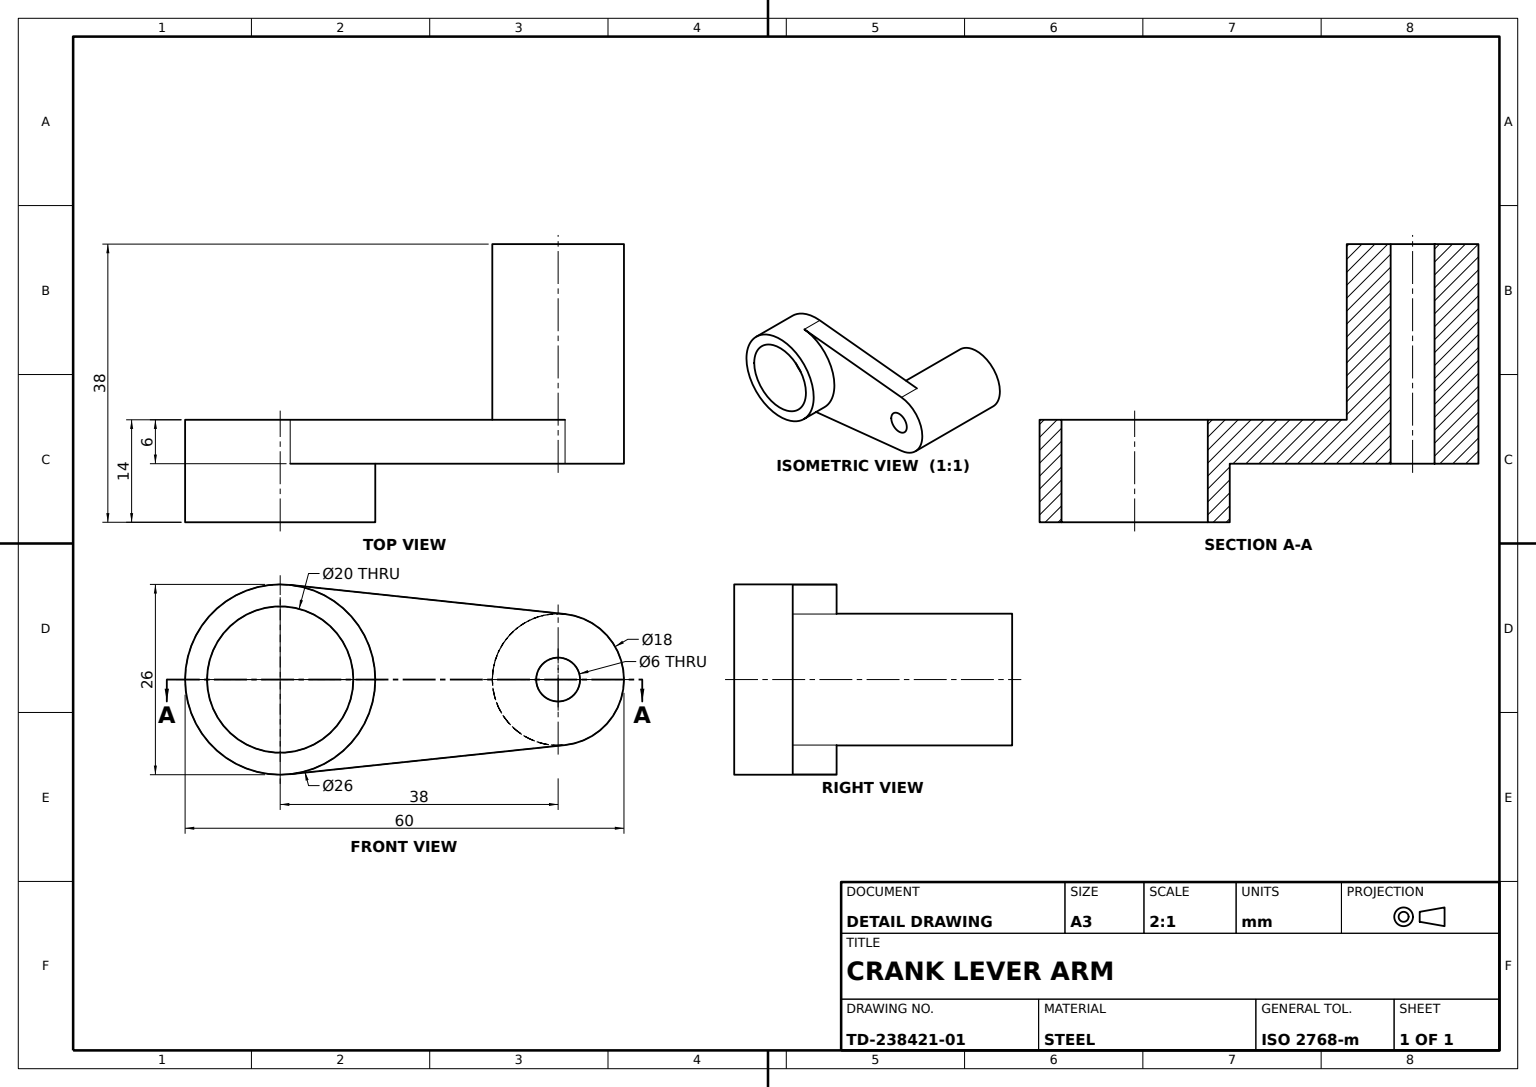
from build123d import *

# Parameters (mm, degrees)
HUB_AND_POST_PROFILE_SKETCH_R   = 13
HUB_AND_POST_PROFILE_SKETCH_R_2 = 10
HUB_RING_26X_20_DEPTH           = 14
SKETCH1_3_R                     = 9
PIN_POST_18_DEPTH               = 24
ARM_WEB_SKETCH_R                = 9
ARM_WEB_6MM_DEPTH               = 6
PIN_HOLE_SKETCH_R               = 3
PIN_HOLE_6_DEPTH                = 37


with BuildPart() as part:
    # Hub and Post Profile Sketch → Hub Ring _26x_20 (new body)
    with BuildSketch(Plane(origin=(0, 0, 0), x_dir=(0, 0, -1), z_dir=(1, 0, 0))):
        Circle(HUB_AND_POST_PROFILE_SKETCH_R)
        Circle(HUB_AND_POST_PROFILE_SKETCH_R_2, mode=Mode.SUBTRACT)
    extrude(amount=HUB_RING_26X_20_DEPTH)



with BuildPart() as body_2:
    # Sketch1_3 → Pin Post _18 (new body)
    with BuildSketch(Plane(origin=(0, 0, 0), x_dir=(0, 0, -1), z_dir=(1, 0, 0))):
        with Locations((38, 0)):
            Circle(SKETCH1_3_R)
    extrude(amount=-PIN_POST_18_DEPTH)


with BuildPart() as part_1:
    add(part.part)

    add(body_2.part)  # Arm Web 6mm merges body 2
    # Arm Web Sketch → Arm Web 6mm (add)
    with BuildSketch(Plane(origin=(0, 0, 0), x_dir=(0, 0, -1), z_dir=(1, 0, 0))):
        with BuildLine():
            Line((38.947368421, 8.949999613), (1.368421053, 12.927777219))
            ThreePointArc((1.368421053, 12.927777219), (9.664095242, 8.695128703), (13, 0))
            ThreePointArc((13, 0), (9.664095242, -8.695128703), (1.368421053, -12.927777219))
            Line((1.368421053, -12.927777219), (38.947368421, -8.949999613))
            ThreePointArc((38.947368421, -8.949999613), (29, 0), (38.947368421, 8.949999613))
        make_face()
        with Locations(Location((38, 0, 0), (0, 0, 276.042328419))):
            Circle(ARM_WEB_SKETCH_R)
    extrude(amount=ARM_WEB_6MM_DEPTH)

    # Pin Hole Sketch → Pin Hole _6 (cut)
    with BuildSketch(Plane(origin=(6, 0, 0), x_dir=(0, 0, -1), z_dir=(1, 0, 0))):
        with Locations((38, 0)):
            Circle(PIN_HOLE_SKETCH_R)
    extrude(amount=-PIN_HOLE_6_DEPTH, mode=Mode.SUBTRACT)


solid = part_1.part
